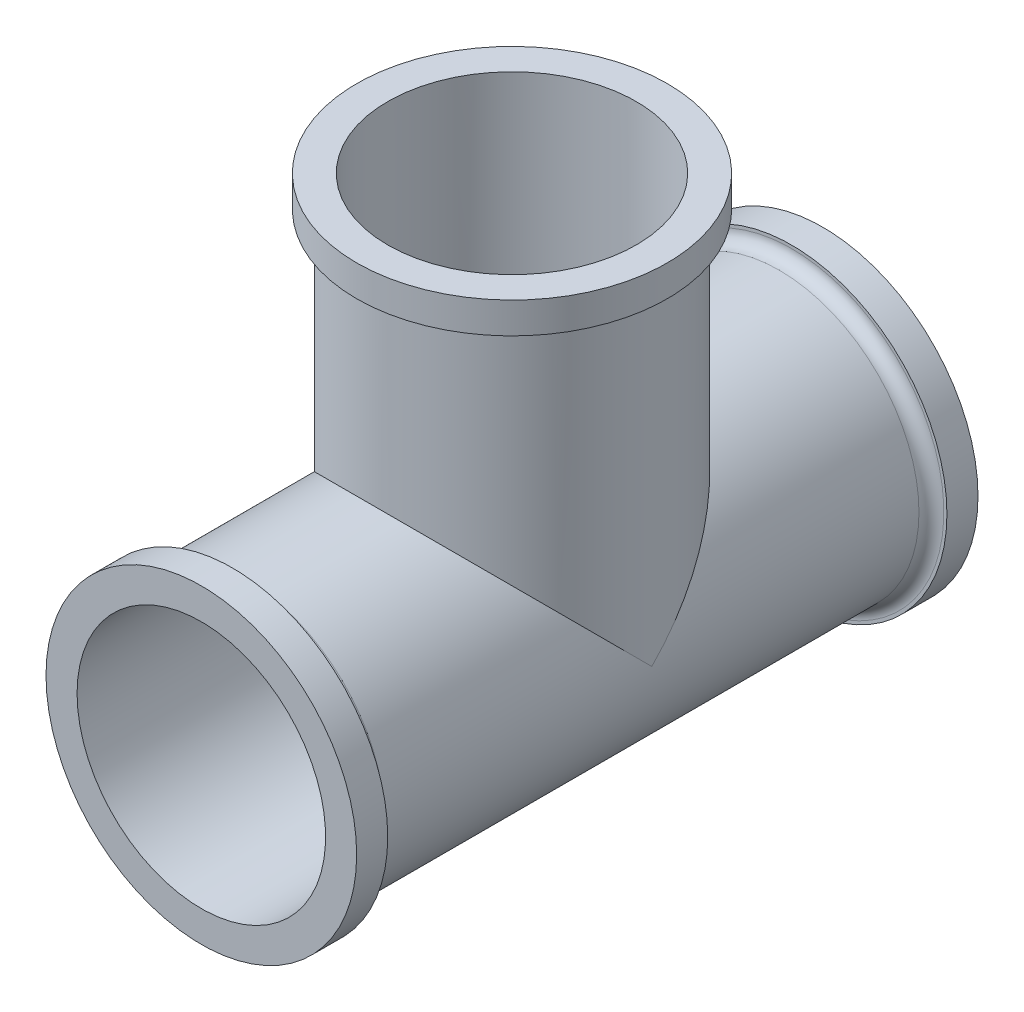
ISO-10303-21;
HEADER;
FILE_DESCRIPTION(('STEP AP214'),'2;1');
FILE_NAME('part.step','',(''),(''),'','','');
FILE_SCHEMA(('AUTOMOTIVE_DESIGN { 1 0 10303 214 1 1 1 1 }'));
ENDSEC;
DATA;
#1=APPLICATION_CONTEXT('core data for automotive mechanical design processes');
#2=APPLICATION_PROTOCOL_DEFINITION('international standard','automotive_design',2000,#1);
#3=PRODUCT_CONTEXT('',#1,'mechanical');
#4=PRODUCT('Part','Part','',(#3));
#5=PRODUCT_RELATED_PRODUCT_CATEGORY('part','',(#4));
#6=PRODUCT_DEFINITION_FORMATION('','',#4);
#7=PRODUCT_DEFINITION_CONTEXT('part definition',#1,'design');
#8=PRODUCT_DEFINITION('design','',#6,#7);
#9=PRODUCT_DEFINITION_SHAPE('','',#8);
#10=(LENGTH_UNIT() NAMED_UNIT(*) SI_UNIT(.MILLI.,.METRE.));
#11=(NAMED_UNIT(*) PLANE_ANGLE_UNIT() SI_UNIT($,.RADIAN.));
#12=(NAMED_UNIT(*) SI_UNIT($,.STERADIAN.) SOLID_ANGLE_UNIT());
#13=UNCERTAINTY_MEASURE_WITH_UNIT(LENGTH_MEASURE(1.E-05),#10,'distance_accuracy_value','');
#14=(GEOMETRIC_REPRESENTATION_CONTEXT(3) GLOBAL_UNCERTAINTY_ASSIGNED_CONTEXT((#13)) GLOBAL_UNIT_ASSIGNED_CONTEXT((#10,
#11,#12)) REPRESENTATION_CONTEXT('',''));
#15=CARTESIAN_POINT('',(0.,0.,0.));
#16=DIRECTION('',(0.,0.,1.));
#17=DIRECTION('',(1.,0.,0.));
#18=AXIS2_PLACEMENT_3D('',#15,#16,#17);
#19=CARTESIAN_POINT('',(0.,27.,-23.75));
#20=DIRECTION('',(0.,-1.,0.));
#21=DIRECTION('',(0.,0.,-1.));
#22=AXIS2_PLACEMENT_3D('',#19,#20,#21);
#23=CYLINDRICAL_SURFACE('',#22,11.25);
#24=CARTESIAN_POINT('',(0.,0.,-23.75));
#25=DIRECTION('',(0.,-0.707106781186548,0.707106781186547));
#26=DIRECTION('',(0.,0.707106781186548,0.707106781186547));
#27=AXIS2_PLACEMENT_3D('',#24,#25,#26);
#28=ELLIPSE('',#27,15.9099025766973,11.25);
#29=CARTESIAN_POINT('',(11.25,0.,-23.75));
#30=VERTEX_POINT('',#29);
#31=CARTESIAN_POINT('',(-11.25,0.,-23.75));
#32=VERTEX_POINT('',#31);
#33=EDGE_CURVE('E61',#30,#32,#28,.T.);
#34=ORIENTED_EDGE('',*,*,#33,.F.);
#35=CARTESIAN_POINT('',(0.,0.,-23.75));
#36=DIRECTION('',(0.,0.707106781186548,0.707106781186547));
#37=DIRECTION('',(0.,-0.707106781186548,0.707106781186547));
#38=AXIS2_PLACEMENT_3D('',#35,#36,#37);
#39=ELLIPSE('',#38,15.9099025766973,11.25);
#40=EDGE_CURVE('E81',#32,#30,#39,.F.);
#41=ORIENTED_EDGE('',*,*,#40,.F.);
#42=EDGE_LOOP('',(#34,#41));
#43=FACE_BOUND('',#42,.T.);
#44=CARTESIAN_POINT('',(0.,26.25,-23.75));
#45=DIRECTION('',(0.,1.,0.));
#46=DIRECTION('',(0.,0.,1.));
#47=AXIS2_PLACEMENT_3D('',#44,#45,#46);
#48=CIRCLE('',#47,11.25);
#49=CARTESIAN_POINT('',(0.,26.25,-12.5));
#50=VERTEX_POINT('',#49);
#51=EDGE_CURVE('E11',#50,#50,#48,.T.);
#52=ORIENTED_EDGE('',*,*,#51,.F.);
#53=EDGE_LOOP('',(#52));
#54=FACE_BOUND('',#53,.T.);
#55=ADVANCED_FACE('F43',(#43,#54),#23,.T.);
#56=CARTESIAN_POINT('',(0.,0.,-46.25));
#57=DIRECTION('',(0.,0.,1.));
#58=DIRECTION('',(1.,0.,0.));
#59=AXIS2_PLACEMENT_3D('',#56,#57,#58);
#60=CYLINDRICAL_SURFACE('',#59,11.25);
#61=CARTESIAN_POINT('',(0.,0.,-2.25));
#62=DIRECTION('',(0.,0.,1.));
#63=DIRECTION('',(1.,0.,0.));
#64=AXIS2_PLACEMENT_3D('',#61,#62,#63);
#65=CIRCLE('',#64,11.25);
#66=CARTESIAN_POINT('',(11.25,0.,-2.25));
#67=VERTEX_POINT('',#66);
#68=EDGE_CURVE('E113',#67,#67,#65,.F.);
#69=ORIENTED_EDGE('',*,*,#68,.T.);
#70=EDGE_LOOP('',(#69));
#71=FACE_BOUND('',#70,.T.);
#72=CARTESIAN_POINT('',(0.,0.,-45.25));
#73=DIRECTION('',(0.,0.,-1.));
#74=DIRECTION('',(-1.,0.,0.));
#75=AXIS2_PLACEMENT_3D('',#72,#73,#74);
#76=CIRCLE('',#75,11.25);
#77=CARTESIAN_POINT('',(-11.25,0.,-45.25));
#78=VERTEX_POINT('',#77);
#79=EDGE_CURVE('E109',#78,#78,#76,.F.);
#80=ORIENTED_EDGE('',*,*,#79,.T.);
#81=EDGE_LOOP('',(#80));
#82=FACE_BOUND('',#81,.T.);
#83=ORIENTED_EDGE('',*,*,#40,.T.);
#84=ORIENTED_EDGE('',*,*,#33,.T.);
#85=EDGE_LOOP('',(#83,#84));
#86=FACE_BOUND('',#85,.T.);
#87=ADVANCED_FACE('F130',(#71,#82,#86),#60,.T.);
#88=CARTESIAN_POINT('',(0.,0.,1.25));
#89=DIRECTION('',(0.,0.,-1.));
#90=DIRECTION('',(-1.,0.,0.));
#91=AXIS2_PLACEMENT_3D('',#88,#89,#90);
#92=CYLINDRICAL_SURFACE('',#91,10.);
#93=CARTESIAN_POINT('',(0.,0.,-23.75));
#94=DIRECTION('',(0.,0.707106781186547,0.707106781186547));
#95=DIRECTION('',(0.,0.707106781186547,-0.707106781186547));
#96=AXIS2_PLACEMENT_3D('',#93,#94,#95);
#97=ELLIPSE('',#96,14.142135623731,10.);
#98=CARTESIAN_POINT('',(-10.,0.,-23.75));
#99=VERTEX_POINT('',#98);
#100=CARTESIAN_POINT('',(10.,0.,-23.75));
#101=VERTEX_POINT('',#100);
#102=EDGE_CURVE('E68',#99,#101,#97,.F.);
#103=ORIENTED_EDGE('',*,*,#102,.F.);
#104=CARTESIAN_POINT('',(0.,0.,-23.75));
#105=DIRECTION('',(0.,0.707106781186547,-0.707106781186547));
#106=DIRECTION('',(0.,0.707106781186547,0.707106781186547));
#107=AXIS2_PLACEMENT_3D('',#104,#105,#106);
#108=ELLIPSE('',#107,14.142135623731,10.);
#109=EDGE_CURVE('E60',#101,#99,#108,.F.);
#110=ORIENTED_EDGE('',*,*,#109,.F.);
#111=EDGE_LOOP('',(#103,#110));
#112=FACE_BOUND('',#111,.T.);
#113=CARTESIAN_POINT('',(0.,0.,-48.75));
#114=DIRECTION('',(0.,0.,-1.));
#115=DIRECTION('',(-1.,0.,0.));
#116=AXIS2_PLACEMENT_3D('',#113,#114,#115);
#117=CIRCLE('',#116,10.);
#118=CARTESIAN_POINT('',(-10.,0.,-48.75));
#119=VERTEX_POINT('',#118);
#120=EDGE_CURVE('E88',#119,#119,#117,.T.);
#121=ORIENTED_EDGE('',*,*,#120,.T.);
#122=EDGE_LOOP('',(#121));
#123=FACE_BOUND('',#122,.T.);
#124=CARTESIAN_POINT('',(0.,0.,1.25));
#125=DIRECTION('',(0.,0.,-1.));
#126=DIRECTION('',(-1.,0.,0.));
#127=AXIS2_PLACEMENT_3D('',#124,#125,#126);
#128=CIRCLE('',#127,10.);
#129=CARTESIAN_POINT('',(-10.,0.,1.25));
#130=VERTEX_POINT('',#129);
#131=EDGE_CURVE('E90',#130,#130,#128,.T.);
#132=ORIENTED_EDGE('',*,*,#131,.F.);
#133=EDGE_LOOP('',(#132));
#134=FACE_BOUND('',#133,.T.);
#135=ADVANCED_FACE('F72',(#112,#123,#134),#92,.F.);
#136=CARTESIAN_POINT('',(0.,0.,1.25));
#137=DIRECTION('',(0.,0.,-1.));
#138=DIRECTION('',(-1.,0.,0.));
#139=AXIS2_PLACEMENT_3D('',#136,#137,#138);
#140=CYLINDRICAL_SURFACE('',#139,12.5);
#141=CARTESIAN_POINT('',(0.,0.,1.25));
#142=DIRECTION('',(0.,0.,1.));
#143=DIRECTION('',(1.,0.,0.));
#144=AXIS2_PLACEMENT_3D('',#141,#142,#143);
#145=CIRCLE('',#144,12.5);
#146=CARTESIAN_POINT('',(12.5,0.,1.25));
#147=VERTEX_POINT('',#146);
#148=EDGE_CURVE('E105',#147,#147,#145,.T.);
#149=ORIENTED_EDGE('',*,*,#148,.F.);
#150=EDGE_LOOP('',(#149));
#151=FACE_BOUND('',#150,.T.);
#152=CARTESIAN_POINT('',(0.,0.,-1.25));
#153=DIRECTION('',(0.,0.,1.));
#154=DIRECTION('',(1.,0.,0.));
#155=AXIS2_PLACEMENT_3D('',#152,#153,#154);
#156=CIRCLE('',#155,12.5);
#157=CARTESIAN_POINT('',(12.5,0.,-1.25));
#158=VERTEX_POINT('',#157);
#159=EDGE_CURVE('E100',#158,#158,#156,.T.);
#160=ORIENTED_EDGE('',*,*,#159,.T.);
#161=EDGE_LOOP('',(#160));
#162=FACE_BOUND('',#161,.T.);
#163=ADVANCED_FACE('F156',(#151,#162),#140,.T.);
#164=CARTESIAN_POINT('',(0.,0.,1.25));
#165=DIRECTION('',(0.,0.,1.));
#166=DIRECTION('',(1.,0.,0.));
#167=AXIS2_PLACEMENT_3D('',#164,#165,#166);
#168=PLANE('',#167);
#169=ORIENTED_EDGE('',*,*,#131,.T.);
#170=EDGE_LOOP('',(#169));
#171=FACE_BOUND('',#170,.T.);
#172=ORIENTED_EDGE('',*,*,#148,.T.);
#173=EDGE_LOOP('',(#172));
#174=FACE_BOUND('',#173,.T.);
#175=ADVANCED_FACE('F166',(#171,#174),#168,.T.);
#176=CARTESIAN_POINT('',(0.,0.,-1.25));
#177=DIRECTION('',(0.,0.,1.));
#178=DIRECTION('',(1.,0.,0.));
#179=AXIS2_PLACEMENT_3D('',#176,#177,#178);
#180=PLANE('',#179);
#181=CARTESIAN_POINT('',(0.,0.,-1.25));
#182=DIRECTION('',(0.,0.,1.));
#183=DIRECTION('',(1.,0.,0.));
#184=AXIS2_PLACEMENT_3D('',#181,#182,#183);
#185=CIRCLE('',#184,12.25);
#186=CARTESIAN_POINT('',(12.25,0.,-1.25));
#187=VERTEX_POINT('',#186);
#188=EDGE_CURVE('E102',#187,#187,#185,.T.);
#189=ORIENTED_EDGE('',*,*,#188,.T.);
#190=EDGE_LOOP('',(#189));
#191=FACE_BOUND('',#190,.T.);
#192=ORIENTED_EDGE('',*,*,#159,.F.);
#193=EDGE_LOOP('',(#192));
#194=FACE_BOUND('',#193,.T.);
#195=ADVANCED_FACE('F164',(#191,#194),#180,.F.);
#196=CARTESIAN_POINT('',(0.,0.,-48.75));
#197=DIRECTION('',(0.,0.,1.));
#198=DIRECTION('',(1.,0.,0.));
#199=AXIS2_PLACEMENT_3D('',#196,#197,#198);
#200=CYLINDRICAL_SURFACE('',#199,12.5);
#201=CARTESIAN_POINT('',(0.,0.,-48.75));
#202=DIRECTION('',(0.,0.,-1.));
#203=DIRECTION('',(-1.,0.,0.));
#204=AXIS2_PLACEMENT_3D('',#201,#202,#203);
#205=CIRCLE('',#204,12.5);
#206=CARTESIAN_POINT('',(-12.5,0.,-48.75));
#207=VERTEX_POINT('',#206);
#208=EDGE_CURVE('E98',#207,#207,#205,.T.);
#209=ORIENTED_EDGE('',*,*,#208,.F.);
#210=EDGE_LOOP('',(#209));
#211=FACE_BOUND('',#210,.T.);
#212=CARTESIAN_POINT('',(0.,0.,-46.25));
#213=DIRECTION('',(0.,0.,-1.));
#214=DIRECTION('',(-1.,0.,0.));
#215=AXIS2_PLACEMENT_3D('',#212,#213,#214);
#216=CIRCLE('',#215,12.5);
#217=CARTESIAN_POINT('',(-12.5,0.,-46.25));
#218=VERTEX_POINT('',#217);
#219=EDGE_CURVE('E92',#218,#218,#216,.T.);
#220=ORIENTED_EDGE('',*,*,#219,.T.);
#221=EDGE_LOOP('',(#220));
#222=FACE_BOUND('',#221,.T.);
#223=ADVANCED_FACE('F159',(#211,#222),#200,.T.);
#224=CARTESIAN_POINT('',(0.,0.,-48.75));
#225=DIRECTION('',(0.,0.,-1.));
#226=DIRECTION('',(-1.,0.,0.));
#227=AXIS2_PLACEMENT_3D('',#224,#225,#226);
#228=PLANE('',#227);
#229=ORIENTED_EDGE('',*,*,#120,.F.);
#230=EDGE_LOOP('',(#229));
#231=FACE_BOUND('',#230,.T.);
#232=ORIENTED_EDGE('',*,*,#208,.T.);
#233=EDGE_LOOP('',(#232));
#234=FACE_BOUND('',#233,.T.);
#235=ADVANCED_FACE('F160',(#231,#234),#228,.T.);
#236=CARTESIAN_POINT('',(0.,0.,-46.25));
#237=DIRECTION('',(0.,0.,-1.));
#238=DIRECTION('',(-1.,0.,0.));
#239=AXIS2_PLACEMENT_3D('',#236,#237,#238);
#240=PLANE('',#239);
#241=CARTESIAN_POINT('',(0.,0.,-46.25));
#242=DIRECTION('',(0.,0.,-1.));
#243=DIRECTION('',(-1.,0.,0.));
#244=AXIS2_PLACEMENT_3D('',#241,#242,#243);
#245=CIRCLE('',#244,12.25);
#246=CARTESIAN_POINT('',(-12.25,0.,-46.25));
#247=VERTEX_POINT('',#246);
#248=EDGE_CURVE('E51',#247,#247,#245,.T.);
#249=ORIENTED_EDGE('',*,*,#248,.T.);
#250=EDGE_LOOP('',(#249));
#251=FACE_BOUND('',#250,.T.);
#252=ORIENTED_EDGE('',*,*,#219,.F.);
#253=EDGE_LOOP('',(#252));
#254=FACE_BOUND('',#253,.T.);
#255=ADVANCED_FACE('F117',(#251,#254),#240,.F.);
#256=CARTESIAN_POINT('',(0.,0.,-2.25));
#257=DIRECTION('',(0.,0.,1.));
#258=DIRECTION('',(1.,0.,0.));
#259=AXIS2_PLACEMENT_3D('',#256,#257,#258);
#260=TOROIDAL_SURFACE('',#259,12.25,1.);
#261=ORIENTED_EDGE('',*,*,#68,.F.);
#262=EDGE_LOOP('',(#261));
#263=FACE_BOUND('',#262,.T.);
#264=ORIENTED_EDGE('',*,*,#188,.F.);
#265=EDGE_LOOP('',(#264));
#266=FACE_BOUND('',#265,.T.);
#267=ADVANCED_FACE('F121',(#263,#266),#260,.F.);
#268=CARTESIAN_POINT('',(0.,0.,-45.25));
#269=DIRECTION('',(0.,0.,-1.));
#270=DIRECTION('',(-1.,0.,0.));
#271=AXIS2_PLACEMENT_3D('',#268,#269,#270);
#272=TOROIDAL_SURFACE('',#271,12.25,1.);
#273=ORIENTED_EDGE('',*,*,#248,.F.);
#274=EDGE_LOOP('',(#273));
#275=FACE_BOUND('',#274,.T.);
#276=ORIENTED_EDGE('',*,*,#79,.F.);
#277=EDGE_LOOP('',(#276));
#278=FACE_BOUND('',#277,.T.);
#279=ADVANCED_FACE('F44',(#275,#278),#272,.F.);
#280=CARTESIAN_POINT('',(0.,28.75,-23.75));
#281=DIRECTION('',(0.,-1.,0.));
#282=DIRECTION('',(0.,0.,-1.));
#283=AXIS2_PLACEMENT_3D('',#280,#281,#282);
#284=CYLINDRICAL_SURFACE('',#283,12.5);
#285=CARTESIAN_POINT('',(0.,28.75,-23.75));
#286=DIRECTION('',(0.,1.,0.));
#287=DIRECTION('',(0.,0.,1.));
#288=AXIS2_PLACEMENT_3D('',#285,#286,#287);
#289=CIRCLE('',#288,12.5);
#290=CARTESIAN_POINT('',(0.,28.75,-11.25));
#291=VERTEX_POINT('',#290);
#292=EDGE_CURVE('E82',#291,#291,#289,.T.);
#293=ORIENTED_EDGE('',*,*,#292,.F.);
#294=EDGE_LOOP('',(#293));
#295=FACE_BOUND('',#294,.T.);
#296=CARTESIAN_POINT('',(0.,26.25,-23.75));
#297=DIRECTION('',(0.,1.,0.));
#298=DIRECTION('',(0.,0.,1.));
#299=AXIS2_PLACEMENT_3D('',#296,#297,#298);
#300=CIRCLE('',#299,12.5);
#301=CARTESIAN_POINT('',(0.,26.25,-11.25));
#302=VERTEX_POINT('',#301);
#303=EDGE_CURVE('E76',#302,#302,#300,.T.);
#304=ORIENTED_EDGE('',*,*,#303,.T.);
#305=EDGE_LOOP('',(#304));
#306=FACE_BOUND('',#305,.T.);
#307=ADVANCED_FACE('F124',(#295,#306),#284,.T.);
#308=CARTESIAN_POINT('',(0.,28.75,0.));
#309=DIRECTION('',(0.,1.,0.));
#310=DIRECTION('',(0.,0.,1.));
#311=AXIS2_PLACEMENT_3D('',#308,#309,#310);
#312=PLANE('',#311);
#313=CARTESIAN_POINT('',(0.,28.75,-23.75));
#314=DIRECTION('',(0.,1.,0.));
#315=DIRECTION('',(0.,0.,1.));
#316=AXIS2_PLACEMENT_3D('',#313,#314,#315);
#317=CIRCLE('',#316,10.);
#318=CARTESIAN_POINT('',(0.,28.75,-13.75));
#319=VERTEX_POINT('',#318);
#320=EDGE_CURVE('E74',#319,#319,#317,.T.);
#321=ORIENTED_EDGE('',*,*,#320,.F.);
#322=EDGE_LOOP('',(#321));
#323=FACE_BOUND('',#322,.T.);
#324=ORIENTED_EDGE('',*,*,#292,.T.);
#325=EDGE_LOOP('',(#324));
#326=FACE_BOUND('',#325,.T.);
#327=ADVANCED_FACE('F139',(#323,#326),#312,.T.);
#328=CARTESIAN_POINT('',(0.,26.25,0.));
#329=DIRECTION('',(0.,1.,0.));
#330=DIRECTION('',(0.,0.,1.));
#331=AXIS2_PLACEMENT_3D('',#328,#329,#330);
#332=PLANE('',#331);
#333=ORIENTED_EDGE('',*,*,#51,.T.);
#334=EDGE_LOOP('',(#333));
#335=FACE_BOUND('',#334,.T.);
#336=ORIENTED_EDGE('',*,*,#303,.F.);
#337=EDGE_LOOP('',(#336));
#338=FACE_BOUND('',#337,.T.);
#339=ADVANCED_FACE('F140',(#335,#338),#332,.F.);
#340=CARTESIAN_POINT('',(0.,-12.501,-23.75));
#341=DIRECTION('',(0.,1.,0.));
#342=DIRECTION('',(0.,0.,1.));
#343=AXIS2_PLACEMENT_3D('',#340,#341,#342);
#344=CYLINDRICAL_SURFACE('',#343,10.);
#345=ORIENTED_EDGE('',*,*,#320,.T.);
#346=EDGE_LOOP('',(#345));
#347=FACE_BOUND('',#346,.T.);
#348=ORIENTED_EDGE('',*,*,#109,.T.);
#349=ORIENTED_EDGE('',*,*,#102,.T.);
#350=EDGE_LOOP('',(#348,#349));
#351=FACE_BOUND('',#350,.T.);
#352=ADVANCED_FACE('F70',(#347,#351),#344,.F.);
#353=CLOSED_SHELL('',(#55,#87,#135,#163,#175,#195,#223,#235,#255,#267,#279,#307,#327,#339,#352));
#354=MANIFOLD_SOLID_BREP('B2',#353);
#355=ADVANCED_BREP_SHAPE_REPRESENTATION('',(#18,#354),#14);
#356=SHAPE_DEFINITION_REPRESENTATION(#9,#355);
ENDSEC;
END-ISO-10303-21;
